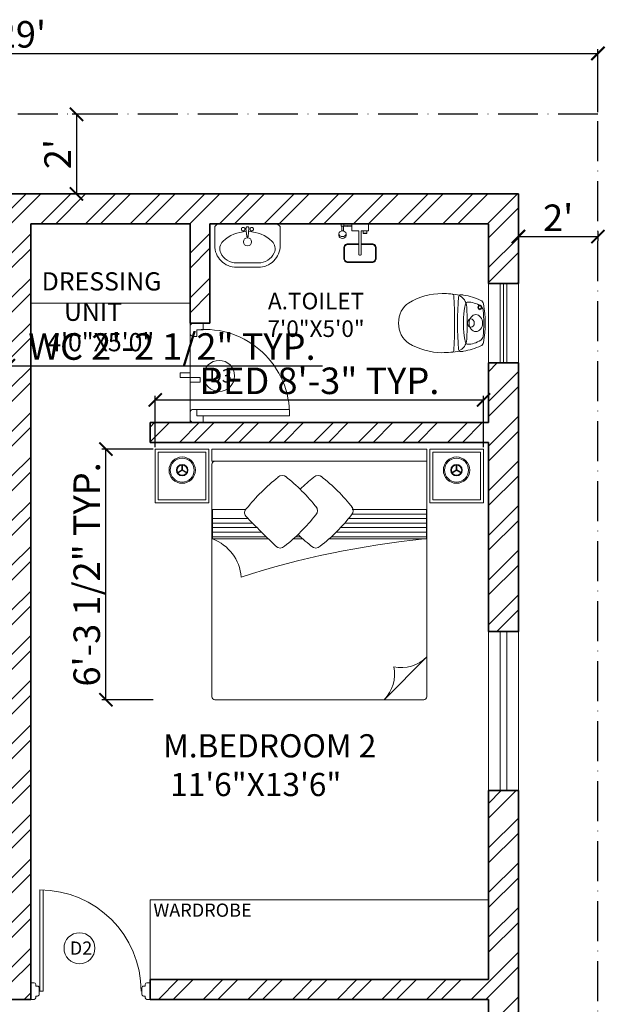
# Model space of a CAD drawing. Units: inches. Extents: x -15 to 1053, y -1 to 793.
# Tile 8 of 8: x 793 to 969, y 496 to 793. Entities that reach past the tile are written whole.
import ezdxf

# ---------------------------------------------------------------- set-up
doc = ezdxf.new("R2010")
doc.units = ezdxf.units.IN
doc.linetypes.add('ACAD_ISO10W100', pattern=[18, 12, -3, 0, -3])
for name, color, linetype, lineweight in [('00 FURNITURE', 15, 'Continuous', 15), ('A-ANNO-DIMS', 2, 'Continuous', 18), ('A-ANNO-TEXT', 7, 'Continuous', 18), ('A-AREA-IDEN', 7, 'Continuous', 18), ('A-DOOR', 4, 'Continuous', 18), ('A-FLOR-CASE', 5, 'Continuous', 18), ('A-FLOR-FIXT', 8, 'Continuous', 13), ('A-FURN', 8, 'Continuous', 13), ('A-GLAZ', 4, 'Continuous', 18), ('A-WALL', 7, 'Continuous', 35), ('A-WALL-PATT', 8, 'Continuous', 13), ('A_FUR 1', 5, 'Continuous', 5), ('C-PROP', 1, 'ACAD_ISO10W100', 25)]:
    doc.layers.add(name, color=color, linetype=linetype, lineweight=lineweight)
doc.styles.add('1-100DIM', font='txt', dxfattribs={"height": 0.3})
doc.styles.get("Standard").update_dxf_attribs({"font": 'arial.ttf'})
doc.dimstyles.new('ISO-25', dxfattribs={"dimtxt": 8, "dimasz": 4, "dimexe": 1.25, "dimexo": 0.625, "dimtad": 1, "dimdec": 0, "dimlunit": 4, "dimtxsty": 'Standard', "dimblk": 'ARCHTICK', "dimcen": 3, "dimadec": 0, "dimazin": 0, "dimtfac": 1, "dimtdec": 0, "dimtmove": 0, "dimatfit": 3, "dimldrblk": 'ARCHTICK', "dimfxl": 1, "dimarcsym": 0})

# ---------------------------------------------------------------- blocks, each defined once
blk = doc.blocks.new('_ArchTick')
at = {"color": 0, "linetype": 'ByBlock', "const_width": 0.15}
blk.add_lwpolyline([(-0.5, -0.5), (0.5, 0.5)], dxfattribs=at)
blk = doc.blocks.new('*D18')
at = {"layer": 'A-ANNO-DIMS', "color": 0, "lineweight": -2, "transparency": 16777216}
for p, q in [((619.07, 765.39), (619.07, 784.39)), ((967.07, 765.39), (967.07, 784.39)), ((619.07, 783.14), (967.07, 783.14))]:
    blk.add_line(p, q, dxfattribs=at)
at = {"layer": 'Defpoints', "color": 0, "transparency": 16777216}
for p in [(967.07, 783.14), (619.07, 764.76), (967.07, 764.76)]:
    blk.add_point(p, dxfattribs=at)
at = {"layer": 'A-ANNO-DIMS', "color": 0, "lineweight": -2, "transparency": 16777216, "xscale": 4, "yscale": 4, "zscale": 4, "rotation": 180}
blk.add_blockref('_ArchTick', (619.07, 783.14), dxfattribs=at)
at = {"layer": 'A-ANNO-DIMS', "color": 0, "lineweight": -2, "transparency": 16777216, "xscale": 4, "yscale": 4, "zscale": 4}
blk.add_blockref('_ArchTick', (967.07, 783.14), dxfattribs=at)
at = {"layer": 'A-ANNO-DIMS', "color": 0, "transparency": 16777216, "insert": (793.07, 787.85), "char_height": 8, "attachment_point": 5}
blk.add_mtext("29'", dxfattribs=at)
blk = doc.blocks.new('ESTSET')
at = {"layer": 'A_FUR 1'}
for p, q in [((-10.44, 4.1), (-10.44, 32.1)), ((-8.44, 4.1), (-8.44, 32.1)), ((-36.44, 6.1), (-36.44, 3.1)), ((-34.44, 6.1), (-36.44, 6.1)), ((-34.44, 4.1), (-34.44, 6.1)), ((-34.44, 4.1), (-34.44, 6.1)), ((-8.44, 4.1), (-8.44, 6.1)), ((-8.44, 6.1), (-6.44, 6.1)), ((-8.44, 4.1), (-8.44, 6.1)), ((-6.44, 6.1), (-6.44, 3.1)), ((-32.44, 4.1), (-34.44, 4.1)), ((-32.44, 4.1), (-34.44, 4.1)), ((-32.44, 3.1), (-32.44, 4.1)), ((-10.44, 3.1), (-10.44, 4.1)), ((-10.44, 4.1), (-8.44, 4.1)), ((-10.44, 4.1), (-8.44, 4.1)), ((-6.44, 2.1), (-36.44, 2.1)), ((-35.44, 2.1), (-33.44, 2.1)), ((-7.44, 2.1), (-9.44, 2.1))]:
    blk.add_line(p, q, dxfattribs=at)
for points in [[(-21.44, 2.1), (-18.67, 2.1), (-18.67, 5.1), (-20.06, 5.1)], [(-20.06, 5.1), (-20.06, -0.91)], [(-21.44, 2.1), (-21.44, -0.91), (-20.06, -0.91)]]:
    blk.add_lwpolyline(points, dxfattribs=at)
for centre, radius, start, end in [((-8.91, 6.46), 25.64, 88.9606, 185.2816), ((-35.44, 3.1), 1, 180, 270), ((-33.44, 3.1), 1, 270, 0), ((-9.44, 3.1), 1, 180, 270), ((-7.44, 3.1), 1, 270, 0)]:
    blk.add_arc(centre, radius, start, end, dxfattribs=at)
blk = doc.blocks.new('DDD')
at = {"layer": '00 FURNITURE'}
for p, q in [((-12579.77, -15859.53), (-12579.77, -15829.05)), ((-12578.77, -15859.53), (-12578.77, -15829.03)), ((-12612.02, -15857.03), (-12612.02, -15862.03)), ((-12611.02, -15857.03), (-12612.02, -15857.03)), ((-12610.52, -15858.03), (-12610.52, -15857.53)), ((-12577.52, -15858.03), (-12577.52, -15857.53)), ((-12577.02, -15857.03), (-12576.02, -15857.03)), ((-12576.02, -15857.03), (-12576.02, -15862.03)), ((-12610.52, -15861.53), (-12610.52, -15861.03)), ((-12578.77, -15859.53), (-12579.77, -15859.53)), ((-12577.52, -15861.53), (-12577.52, -15861.03)), ((-12612.02, -15862.03), (-12611.02, -15862.03)), ((-12576.02, -15862.03), (-12577.02, -15862.03))]:
    blk.add_line(p, q, dxfattribs=at)
for points in [[(-12610.52, -15861.03), (-12610.02, -15861.03, 0.414214), (-12609.52, -15860.53), (-12609.52, -15858.53, 0.414214), (-12610.02, -15858.03), (-12610.52, -15858.03)], [(-12577.52, -15861.03), (-12578.02, -15861.03, -0.414214), (-12578.52, -15860.53), (-12578.52, -15858.53, -0.414214), (-12578.02, -15858.03), (-12577.52, -15858.03)]]:
    blk.add_lwpolyline(points, format="xyb", dxfattribs=at)
for centre, radius, start, end in [((-12578.77, -15859.53), 30.5, 90, 180), ((-12611.02, -15857.53), 0.5, 0, 90), ((-12577.02, -15857.53), 0.5, 90, 180), ((-12611.02, -15861.53), 0.5, 270, 0), ((-12577.02, -15861.53), 0.5, 180, 270)]:
    blk.add_arc(centre, radius, start, end, dxfattribs=at)
blk = doc.blocks.new('RGWTG')
at = {"layer": '00 FURNITURE'}
for p, q in [((578.23, 3473.51), (577.36, 3475.01)), ((578.23, 3473.58), (577.36, 3472.08)), ((578.36, 3473.58), (577.49, 3475.09)), ((578.36, 3473.51), (577.49, 3472)), ((578.29, 3473.62), (580.03, 3473.62)), ((578.29, 3473.47), (580.03, 3473.47)), ((521.93, 3464.58), (509.03, 3451.68)), ((509.03, 3422.63), (509.03, 3463.68)), ((509.93, 3464.58), (566.4, 3464.58)), ((557.53, 3463.84), (557.53, 3464.49)), ((557.53, 3464.49), (566.4, 3464.49)), ((558.2, 3464.49), (558.2, 3435.82)), ((559.57, 3464.49), (559.57, 3437.25)), ((560.94, 3464.49), (560.94, 3438.58)), ((562.3, 3464.49), (562.3, 3439.83)), ((563.67, 3464.49), (563.67, 3440.99)), ((565.04, 3464.49), (565.04, 3442.08)), ((566.4, 3464.58), (580.98, 3464.58)), ((566.4, 3464.49), (566.4, 3442.08)), ((566.4, 3464.49), (566.4, 3463.84)), ((580.98, 3464.58), (580.98, 3416.72)), ((558.2, 3426.48), (558.2, 3425.04)), ((509.03, 3400.68), (509.03, 3422.63)), ((558.2, 3416.13), (558.2, 3399.95)), ((580.98, 3416.72), (580.98, 3400.68)), ((559.57, 3414.75), (559.57, 3399.95)), ((560.94, 3413.39), (560.94, 3399.95)), ((562.3, 3412.04), (562.3, 3399.95)), ((563.67, 3410.72), (563.67, 3399.95)), ((580.08, 3399.78), (509.93, 3399.78)), ((557.53, 3399.95), (557.53, 3400.6)), ((566.4, 3399.95), (557.53, 3399.95)), ((566.4, 3400.6), (566.4, 3399.95)), ((578.23, 3390.78), (577.36, 3392.29)), ((578.36, 3390.86), (577.49, 3392.36)), ((578.23, 3390.86), (577.36, 3389.36)), ((578.36, 3390.78), (577.49, 3389.28)), ((578.29, 3390.9), (580.03, 3390.9)), ((578.29, 3390.74), (580.03, 3390.74))]:
    blk.add_line(p, q, dxfattribs=at)
for points in [[(568.43, 3465.48), (584.63, 3465.48), (584.63, 3481.68), (568.43, 3481.68)], [(569.33, 3466.38), (583.73, 3466.38), (583.73, 3480.78), (569.33, 3480.78)], [(580.98, 3399.78), (584.63, 3399.78), (584.63, 3464.58), (580.98, 3464.58)], [(568.43, 3398.88), (584.63, 3398.88), (584.63, 3382.68), (568.43, 3382.68)], [(569.33, 3397.98), (583.73, 3397.98), (583.73, 3383.58), (569.33, 3383.58)]]:
    blk.add_lwpolyline(points, close=True, dxfattribs=at)
for points in [[(566.52, 3464.49), (557.53, 3464.49), (557.53, 3435.08)], [(557.53, 3427.21), (557.53, 3424.3)], [(557.53, 3416.82), (557.53, 3399.95), (566.4, 3399.95), (566.4, 3409.94)]]:
    blk.add_lwpolyline(points, dxfattribs=at)
for centre, radius in [((578.29, 3473.54), 3.97), ((578.29, 3473.54), 3.63), ((578.29, 3473.54), 1.74), ((578.29, 3473.54), 1.56), ((578.29, 3390.82), 3.97), ((578.29, 3390.82), 3.63), ((578.29, 3390.82), 1.74), ((578.29, 3390.82), 1.56)]:
    blk.add_circle(centre, radius, dxfattribs=at)
for centre, radius, start, end in [((509.93, 3463.68), 0.9, 90, 180), ((529.65, 3456.88), 10.9, 135.0361, 191.9278), ((290.56, 3490.52), 268.3, 342.2214, 354.2925), ((516.73, 3443.97), 10.9, 78.0722, 134.9639), ((598.15, 3399.01), 54.32, 127.931, 142.069), ((566.05, 3440.57), 1.82, 45, 135), ((533.58, 3399.31), 54.32, 37.931, 52.069), ((556.59, 3431.11), 1.82, 135, 225), ((598.15, 3388.23), 54.32, 127.931, 142.069), ((566.05, 3429.78), 1.82, 45, 135), ((533.58, 3388.53), 54.32, 37.931, 52.069), ((574.84, 3431.77), 1.82, 315, 45), ((597.87, 3463.6), 54.32, 217.931, 224.141), ((533.28, 3463.88), 54.32, 316.32, 322.069), ((574.84, 3420.99), 1.82, 315, 45), ((556.59, 3420.33), 1.82, 135, 225), ((765.33, 3619.75), 290.45, 223.6069, 226.2326), ((533.28, 3453.1), 54.32, 307.931, 322.069), ((565.44, 3411.05), 1.47, 225.9674, 326.8337), ((545.02, 3395.29), 13.35, 20.4224, 85.5825), ((509.93, 3400.68), 0.9, 180, 270), ((580.08, 3400.68), 0.9, 270, 0)]:
    blk.add_arc(centre, radius, start, end, dxfattribs=at)
blk = doc.blocks.new('s_14')
at = {"extrusion": (0, 0, -1)}
for centre, major_axis, start_param, end_param in [((-0.2, -522.3), (652.4, -0.3), 4.476887, 4.947891), ((-0.2, -522.3), (652.4, -0.3), 4.476887, 4.947891), ((681.3, -278.7), (913.7, -0.4), 3.289642, 3.481728), ((681.3, -278.7), (913.7, -0.4), 3.289642, 3.481728), ((-143.1, -44.8), (39.1, 0), 3.481728, 4.476887), ((-143.1, -44.8), (39.1, 0), 3.481728, 4.476887), ((118.1, -139.4), (284.9, -0.1), 3.130806, 3.616946), ((-125.1, -42.1), (19.2, 0), 3.141593, 9.424778), ((-125.1, -42.1), (12.2, 0), 3.141593, 9.424778), ((-97.4, -50.5), (42.5, 0), 3.616946, 4.577347), ((-0.3, -624.1), (765.5, -0.4), 4.577347, 4.847431), ((0, -73.8), (67.1, 0), 3.141593, 9.424778), ((97.3, -50.6), (42.5, 0), -1.435755, -0.475353), ((-118.3, -139.3), (284.9, -0.1), -0.475353, 0.010787), ((143.1, -44.9), (39.1, 0), -1.335294, -0.340135), ((143.1, -44.9), (39.1, 0), -1.335294, -0.340135), ((-681.5, -278.1), (913.7, -0.4), -0.340135, -0.148049), ((-681.5, -278.1), (913.7, -0.4), -0.340135, -0.148049), ((-120.9, -224.6), (98.7, 0), 3.365215, 4.657014), ((-148.9, -141.6), (17.9, 0), 1.839297, 3.130806), ((0.1, 291.4), (579, -0.3), 1.302296, 1.839297), ((-0.9, -1969.6), (2281.8, -1.1), 4.657014, 4.767764), ((-0.1, -112.6), (32.9, 0), 3.141593, 9.424778), ((120.7, -224.8), (98.7, 0), -1.515421, -0.223622), ((148.8, -141.7), (17.9, 0), 0.010787, 1.302296), ((999.2, -341.8), (1233.1, -0.6), 3.141593, 3.282422), ((999.2, -341.8), (1233.1, -0.6), 3.141593, 3.282422), ((-87.1, -186.6), (136.8, -0.1), 3.032389, 3.289642), ((-87.1, -186.6), (136.8, -0.1), 3.032389, 3.289642), ((-207.2, -197.1), (16, 0), 1.680926, 3.032389), ((-207.2, -197.1), (16, 0), 1.680926, 3.032389), ((0.6, 1302.1), (1900.3, -0.9), 1.460666, 1.680926), ((0.6, 1302.1), (1900.3, -0.9), 1.460666, 1.680926), ((207, -197.3), (16, 0), 0.109204, 1.460666), ((207, -197.3), (16, 0), 0.109204, 1.460666), ((-999.6, -340.9), (1233.1, -0.6), -0.140829, 0), ((-999.6, -340.9), (1233.1, -0.6), -0.140829, 0), ((86.9, -186.7), (136.8, -0.1), -0.148049, 0.109204), ((86.9, -186.7), (136.8, -0.1), -0.148049, 0.109204), ((-210, -262.6), (19.7, 0), 3.222651, 4.658459), ((-1.6, -3375.8), (3914.3, -1.8), 4.658459, 4.766319), ((209.8, -262.8), (19.7, 0), -1.516867, -0.081058), ((526.7, -341.6), (760.5, -0.4), 2.693443, 3.141593), ((526.7, -341.6), (760.5, -0.4), 2.693443, 3.141593), ((-527, -341.1), (760.5, -0.4), 0, 0.44815), ((-527, -341.1), (760.5, -0.4), 0, 0.44815), ((-0.3, -544.1), (175.9, -0.1), 0.44815, 2.693443), ((-0.3, -544.1), (175.9, -0.1), 0.44815, 2.693443)]:
    blk.add_ellipse(centre, major_axis=major_axis, ratio=0.800511, start_param=start_param, end_param=end_param, dxfattribs=at)
blk = doc.blocks.new('s_46')
at = {"ltscale": 600}
h = blk.add_hatch(color=256, dxfattribs=at)
edge = h.paths.add_edge_path()
edge.add_line((13.5, 62), (14.2, 54.1))
edge.add_ellipse((4.2, 52.3), major_axis=(-10.1, 0), ratio=1, start_angle=540, end_angle=550.17546, ccw=False)
edge.add_arc((4.2, 52.3), 10.1, 270, 360, ccw=False)
edge.add_line((4.2, 42.2), (4.2, 41.3))
edge.add_line((4.2, 41.3), (11.9, 41.3))
edge.add_arc((4.2, 52.3), 13.4, 664.69813, 766.48477)
h.paths.add_polyline_path([(4.2, 41.3), (-3.4, 41.3, 0.152567), (4.2, 38.9)])
h.paths.add_polyline_path([(11.9, 41.3), (4.2, 41.3), (4.2, 38.9, 0.152567)])
h.paths.add_polyline_path([(-5.7, 54.1), (-5, 62, 0.475833), (-3.4, 41.3), (4.2, 41.3), (4.2, 42.2, -0.46724)])
for p, q in [((-5.9, 52.3), (-0.7, 110.5)), ((-5.9, 52.3), (-0.7, 110.5)), ((9.1, 110.5), (14.2, 54.1)), ((14.3, 52.3), (9.1, 110.5)), ((14.2, 54.1), (14.3, 52.3))]:
    blk.add_line(p, q, dxfattribs=at)
blk.add_lwpolyline([(-220.8, 171.3, -0.414214), (-70.8, 321.3), (79.2, 321.3, -0.414214), (229.2, 171.3), (229.2, 41.3), (209.2, 21.3), (-200.8, 21.3), (-220.8, 41.3)], format="xyb", close=True, dxfattribs=at)
blk.add_lwpolyline([(12.3, 75.4, 0.181638), (172.2, 141.5, 0.326351), (187.7, 222.7, 0.289814), (79.2, 291.3), (-70.8, 291.3, 0.289814), (-179.2, 222.7, 0.326351), (-163.8, 141.5, 0.181638), (-3.8, 75.4)], format="xyb", dxfattribs=at)
for points in [[(-16.8, 67.4), (-17, 67.5), (-17.2, 67.6), (-17.4, 67.6), (-17.6, 67.7), (-17.8, 67.8), (-18, 67.9), (-18.1, 68.1), (-18.2, 68.2), (-18.3, 68.4), (-18.4, 68.6), (-18.5, 68.8), (-18.7, 68.9), (-18.8, 69.1), (-18.9, 69.2), (-19.1, 69.3), (-19.3, 69.3), (-19.5, 69.3), (-19.7, 69.4), (-19.9, 69.4), (-20.1, 69.4), (-20.3, 69.4), (-20.5, 69.5), (-20.7, 69.6), (-20.8, 69.7), (-21, 69.9), (-21.1, 70), (-21.3, 70.2), (-21.4, 70.3), (-21.5, 70.4), (-21.7, 70.5), (-21.9, 70.5), (-22.1, 70.5), (-22.3, 70.5), (-22.5, 70.5), (-22.7, 70.4), (-22.9, 70.4), (-23.1, 70.4), (-23.3, 70.4), (-23.5, 70.5), (-23.7, 70.6), (-23.9, 70.7), (-24, 70.8), (-24.2, 70.9), (-24.4, 71), (-24.6, 71.1), (-24.7, 71.1), (-24.9, 71.1), (-25.1, 71), (-25.3, 71), (-25.5, 70.9), (-25.7, 70.8), (-25.9, 70.7), (-26.1, 70.6), (-26.3, 70.6), (-26.5, 70.6), (-26.7, 70.6), (-26.9, 70.7), (-27.1, 70.8), (-27.3, 70.8), (-27.5, 70.9), (-27.7, 70.9), (-27.8, 70.9), (-28, 70.8), (-28.2, 70.8), (-28.3, 70.6), (-28.5, 70.5), (-28.7, 70.4), (-28.9, 70.3), (-29.1, 70.2), (-29.3, 70.1), (-29.6, 70.1), (-29.9, 70.1), (-30.2, 70.1), (-30.5, 70), (-30.8, 69.8), (-31.1, 69.5), (-31.4, 69), (-31.6, 68.4), (-32.3, 68.5), (-32.8, 68.4), (-33.2, 68.3), (-33.5, 68.1), (-33.7, 67.8), (-33.9, 67.6), (-34, 67.3), (-34.1, 67.1), (-34.3, 66.9), (-34.5, 66.7), (-34.7, 66.6), (-34.9, 66.5), (-35.1, 66.4), (-35.2, 66.3), (-35.4, 66.2), (-35.5, 66), (-35.6, 65.9), (-35.6, 65.7), (-35.7, 65.5), (-35.7, 65.3), (-35.7, 65.1), (-35.8, 64.9), (-35.8, 64.7), (-35.9, 64.5), (-36, 64.3), (-36.2, 64.2), (-36.3, 64), (-36.5, 63.9), (-36.6, 63.8), (-36.8, 63.6), (-36.9, 63.5), (-37, 63.3), (-37, 63.1), (-37, 63), (-37, 62.8), (-37, 62.6), (-37, 62.3), (-37, 62.1), (-37, 61.9), (-37, 61.7), (-37.1, 61.5), (-37.2, 61.4), (-37.3, 61.2), (-37.4, 61), (-37.5, 60.8), (-37.6, 60.7), (-37.7, 60.5), (-37.8, 60.3), (-37.8, 60.1), (-37.7, 60), (-37.7, 59.8), (-37.6, 59.6), (-37.5, 59.4), (-37.4, 59.2), (-37.4, 59), (-37.4, 58.8), (-37.4, 58.6), (-37.4, 58.4), (-37.5, 58.2), (-37.6, 58), (-37.7, 57.8), (-37.7, 57.6), (-37.8, 57.4), (-37.8, 57.2), (-37.7, 57.1), (-37.6, 56.9), (-37.5, 56.7), (-37.4, 56.6), (-37.3, 56.4), (-37.2, 56.2), (-37.1, 56), (-37, 55.8), (-37, 55.6), (-37, 55.4), (-37, 55.2), (-37, 55), (-37, 54.8), (-37, 54.6), (-37, 54.4), (-37, 54.2), (-36.9, 54.1), (-36.8, 53.9), (-36.6, 53.8), (-36.5, 53.7), (-36.3, 53.5), (-36.2, 53.4), (-36, 53.2), (-35.9, 53.1), (-35.8, 52.9), (-35.8, 52.7), (-35.7, 52.5), (-35.7, 52.3), (-35.7, 52.1), (-35.6, 51.9), (-35.6, 51.7), (-35.5, 51.5), (-35.4, 51.4), (-35.2, 51.3), (-35.1, 51.2), (-34.9, 51.1), (-34.7, 51), (-34.5, 50.9), (-34.3, 50.8), (-34.2, 50.7), (-34, 50.5), (-33.9, 50.3), (-33.8, 50.1), (-33.8, 49.9), (-33.7, 49.8), (-33.6, 49.6), (-33.5, 49.4), (-33.4, 49.3), (-33.2, 49.2), (-33.1, 49.1), (-32.9, 49.1), (-32.7, 49), (-32.5, 49), (-32.2, 48.9), (-32.1, 48.9), (-31.9, 48.8), (-31.7, 48.7), (-31.6, 48.5), (-31.4, 48.3), (-31.3, 48.2), (-31.2, 48), (-31.1, 47.9), (-30.9, 47.7), (-30.8, 47.6), (-30.6, 47.6), (-30.4, 47.5), (-30.2, 47.5), (-30, 47.6), (-29.8, 47.6), (-29.6, 47.6), (-29.4, 47.6), (-29.2, 47.5), (-29, 47.4), (-28.8, 47.3), (-28.7, 47.2), (-28.5, 47.1), (-28.3, 46.9), (-28.2, 46.8), (-28, 46.7), (-27.8, 46.7), (-27.7, 46.7), (-27.5, 46.7), (-27.3, 46.7), (-27.1, 46.8), (-26.9, 46.9), (-26.7, 46.9), (-26.5, 47), (-26.3, 47), (-26.1, 46.9), (-25.9, 46.9), (-25.7, 46.8), (-25.5, 46.7), (-25.3, 46.6), (-25.1, 46.5), (-24.9, 46.5), (-24.7, 46.5), (-24.6, 46.5), (-24.4, 46.6), (-24.2, 46.7), (-24, 46.8), (-23.9, 46.9), (-23.7, 47), (-23.5, 47.1), (-23.3, 47.1), (-23.1, 47.2), (-22.9, 47.2), (-22.7, 47.1), (-22.5, 47.1), (-22.3, 47), (-22.1, 47), (-21.9, 47), (-21.7, 47.1), (-21.5, 47.1), (-21.4, 47.2), (-21.3, 47.4), (-21.1, 47.5), (-21, 47.7), (-20.8, 47.8), (-20.7, 48), (-20.5, 48.1), (-20.3, 48.1), (-20.1, 48.2), (-19.9, 48.2), (-19.7, 48.2), (-19.5, 48.2), (-19.3, 48.2), (-19.1, 48.3), (-18.9, 48.4), (-18.8, 48.5), (-18.7, 48.6), (-18.5, 48.8), (-18.4, 49), (-18.3, 49.2), (-18.2, 49.3), (-18.1, 49.5), (-18, 49.7), (-17.8, 49.8), (-17.6, 49.9), (-17.4, 49.9), (-17.2, 50), (-17, 50.1), (-16.8, 50.1), (-16.7, 50.2), (-16.5, 50.3), (-16.4, 50.5), (-16.3, 50.7), (-16.3, 50.8), (-16.2, 51), (-16.2, 51.3), (-16.1, 51.5), (-16, 51.6), (-15.9, 51.8), (-15.8, 52), (-15.6, 52.1), (-15.5, 52.2), (-15.3, 52.3), (-15.1, 52.4), (-15, 52.6), (-14.8, 52.7), (-14.7, 52.8), (-14.7, 53), (-14.6, 53.2), (-14.6, 53.4), (-14.6, 53.6), (-14.6, 53.8), (-14.6, 54), (-14.6, 54.2), (-14.5, 54.4), (-14.4, 54.6), (-14.3, 54.8), (-14.2, 54.9), (-14, 55.1), (-13.9, 55.2), (-13.7, 55.4), (-13.6, 55.5), (-13.6, 55.7), (-13.6, 55.9), (-13.6, 56.1), (-13.6, 56.3), (-13.7, 56.5), (-13.7, 56.7), (-13.8, 56.9), (-13.8, 57.1), (-13.8, 57.3), (-13.7, 57.5), (-13.7, 57.7), (-13.6, 57.9), (-13.5, 58.1), (-13.4, 58.2), (-13.3, 58.4), (-13.2, 58.6), (-13.2, 58.8), (-13.2, 59), (-13.3, 59.1), (-13.4, 59.3), (-13.5, 59.5), (-13.6, 59.7), (-13.7, 59.9), (-13.7, 60.1), (-13.8, 60.3), (-13.8, 60.5), (-13.8, 60.7), (-13.7, 60.9), (-13.7, 61.1), (-13.6, 61.3), (-13.6, 61.5), (-13.6, 61.7), (-13.6, 61.9), (-13.6, 62), (-13.7, 62.2), (-13.9, 62.3), (-14, 62.5), (-14.2, 62.6), (-14.3, 62.8), (-14.4, 63), (-14.5, 63.1), (-14.6, 63.3), (-14.6, 63.5), (-14.6, 63.8), (-14.6, 64), (-14.6, 64.2), (-14.6, 64.4), (-14.7, 64.6), (-14.7, 64.7), (-14.8, 64.9), (-15, 65), (-15.1, 65.1), (-15.3, 65.2), (-15.5, 65.3), (-15.6, 65.5), (-15.8, 65.6), (-15.9, 65.7), (-16, 65.9), (-16.1, 66.1), (-16.2, 66.3), (-16.2, 66.5), (-16.3, 66.7), (-16.3, 66.9), (-16.4, 67.1), (-16.5, 67.2), (-16.7, 67.3)], [(22.1, 61.1), (22, 61.3), (22, 61.5), (22, 61.7), (22, 61.9), (22.1, 62), (22.2, 62.2), (22.3, 62.3), (22.4, 62.5), (22.6, 62.6), (22.7, 62.8), (22.8, 63), (22.9, 63.1), (23, 63.3), (23, 63.5), (23, 63.8), (23, 64), (23, 64.2), (23, 64.4), (23.1, 64.6), (23.1, 64.7), (23.2, 64.9), (23.4, 65), (23.5, 65.1), (23.7, 65.2), (23.9, 65.3), (24.1, 65.5), (24.2, 65.6), (24.4, 65.7), (24.5, 65.9), (24.5, 66.1), (24.6, 66.3), (24.7, 66.5), (24.7, 66.7), (24.8, 66.9), (24.9, 67.1), (25, 67.2), (25.1, 67.3), (25.3, 67.4), (25.4, 67.5), (25.6, 67.6), (25.8, 67.6), (26, 67.7), (26.2, 67.8), (26.4, 67.9), (26.5, 68.1), (26.7, 68.2), (26.8, 68.4), (26.9, 68.6), (27, 68.8), (27.1, 68.9), (27.2, 69.1), (27.3, 69.2), (27.5, 69.3), (27.7, 69.3), (27.9, 69.3), (28.1, 69.4), (28.3, 69.4), (28.5, 69.4), (28.7, 69.4), (28.9, 69.5), (29.1, 69.6), (29.2, 69.7), (29.4, 69.9), (29.5, 70), (29.7, 70.2), (29.8, 70.3), (30, 70.4), (30.1, 70.5), (30.3, 70.5), (30.5, 70.5), (30.7, 70.5), (30.9, 70.5), (31.1, 70.4), (31.3, 70.4), (31.5, 70.4), (31.7, 70.4), (31.9, 70.5), (32.1, 70.6), (32.3, 70.7), (32.5, 70.8), (32.6, 70.9), (32.8, 71), (33, 71.1), (33.2, 71.1), (33.4, 71.1), (33.5, 71), (33.7, 71), (33.9, 70.9), (34.1, 70.8), (34.3, 70.7), (34.5, 70.6), (34.7, 70.6), (34.9, 70.6), (35.1, 70.6), (35.3, 70.7), (35.5, 70.8), (35.7, 70.8), (35.9, 70.9), (36.1, 70.9), (36.3, 70.9), (36.4, 70.8), (36.6, 70.8), (36.8, 70.6), (36.9, 70.5), (37.1, 70.4), (37.3, 70.3), (37.5, 70.2), (37.8, 70.1), (38, 70.1), (38.3, 70.1), (38.6, 70.1), (38.9, 70), (39.2, 69.8), (39.5, 69.5), (39.8, 69), (40.1, 68.4), (40.7, 68.5), (41.3, 68.4), (41.7, 68.3), (42, 68.1), (42.2, 67.8), (42.3, 67.6), (42.4, 67.3), (42.6, 67.1), (42.7, 66.9), (42.9, 66.7), (43.1, 66.6), (43.3, 66.5), (43.5, 66.4), (43.6, 66.3), (43.8, 66.2), (43.9, 66), (44, 65.9), (44.1, 65.7), (44.1, 65.5), (44.1, 65.3), (44.2, 65.1), (44.2, 64.9), (44.2, 64.7), (44.3, 64.5), (44.4, 64.3), (44.6, 64.2), (44.7, 64), (44.9, 63.9), (45.1, 63.8), (45.2, 63.6), (45.3, 63.5), (45.4, 63.3), (45.5, 63.1), (45.5, 63), (45.5, 62.8), (45.4, 62.6), (45.4, 62.3), (45.4, 62.1), (45.4, 61.9), (45.4, 61.7), (45.5, 61.5), (45.6, 61.4), (45.7, 61.2), (45.8, 61), (46, 60.8), (46.1, 60.7), (46.1, 60.5), (46.2, 60.3), (46.2, 60.1), (46.1, 60), (46.1, 59.8), (46, 59.6), (45.9, 59.4), (45.9, 59.2), (45.8, 59), (45.8, 58.8), (45.8, 58.6), (45.9, 58.4), (45.9, 58.2), (46, 58), (46.1, 57.8), (46.1, 57.6), (46.2, 57.4), (46.2, 57.2), (46.1, 57.1), (46.1, 56.9), (46, 56.7), (45.8, 56.6), (45.7, 56.4), (45.6, 56.2), (45.5, 56), (45.4, 55.8), (45.4, 55.6), (45.4, 55.4), (45.4, 55.2), (45.4, 55), (45.5, 54.8), (45.5, 54.6), (45.5, 54.4), (45.4, 54.2), (45.3, 54.1), (45.2, 53.9), (45.1, 53.8), (44.9, 53.7), (44.7, 53.5), (44.6, 53.4), (44.4, 53.2), (44.3, 53.1), (44.2, 52.9), (44.2, 52.7), (44.2, 52.5), (44.1, 52.3), (44.1, 52.1), (44.1, 51.9), (44, 51.7), (43.9, 51.5), (43.8, 51.4), (43.6, 51.3), (43.5, 51.2), (43.3, 51.1), (43.1, 51), (42.9, 50.9), (42.7, 50.8), (42.6, 50.7), (42.5, 50.5), (42.4, 50.3), (42.3, 50.1), (42.2, 49.9), (42.1, 49.8), (42, 49.6), (41.9, 49.4), (41.8, 49.3), (41.7, 49.2), (41.5, 49.1), (41.3, 49.1), (41.1, 49), (40.9, 49), (40.7, 48.9), (40.5, 48.9), (40.3, 48.8), (40.1, 48.7), (40, 48.5), (39.9, 48.3), (39.7, 48.2), (39.6, 48), (39.5, 47.9), (39.4, 47.7), (39.2, 47.6), (39, 47.6), (38.8, 47.5), (38.6, 47.5), (38.4, 47.6), (38.2, 47.6), (38, 47.6), (37.8, 47.6), (37.6, 47.5), (37.4, 47.4), (37.2, 47.3), (37.1, 47.2), (36.9, 47.1), (36.8, 46.9), (36.6, 46.8), (36.4, 46.7), (36.3, 46.7), (36.1, 46.7), (35.9, 46.7), (35.7, 46.7), (35.5, 46.8), (35.3, 46.9), (35.1, 46.9), (34.9, 47), (34.7, 47), (34.5, 46.9), (34.3, 46.9), (34.1, 46.8), (33.9, 46.7), (33.7, 46.6), (33.5, 46.5), (33.4, 46.5), (33.2, 46.5), (33, 46.5), (32.8, 46.6), (32.6, 46.7), (32.5, 46.8), (32.3, 46.9), (32.1, 47), (31.9, 47.1), (31.7, 47.1), (31.5, 47.2), (31.3, 47.2), (31.1, 47.1), (30.9, 47.1), (30.7, 47), (30.5, 47), (30.3, 47), (30.1, 47.1), (30, 47.1), (29.8, 47.2), (29.7, 47.4), (29.5, 47.5), (29.4, 47.7), (29.2, 47.8), (29.1, 48), (28.9, 48.1), (28.7, 48.1), (28.5, 48.2), (28.3, 48.2), (28.1, 48.2), (27.9, 48.2), (27.7, 48.2), (27.5, 48.3), (27.3, 48.4), (27.2, 48.5), (27.1, 48.6), (27, 48.8), (26.9, 49), (26.8, 49.2), (26.7, 49.3), (26.5, 49.5), (26.4, 49.7), (26.2, 49.8), (26, 49.9), (25.8, 49.9), (25.6, 50), (25.4, 50.1), (25.3, 50.1), (25.1, 50.2), (25, 50.3), (24.9, 50.5), (24.8, 50.7), (24.7, 50.8), (24.7, 51), (24.6, 51.3), (24.5, 51.5), (24.5, 51.6), (24.4, 51.8), (24.2, 52), (24.1, 52.1), (23.9, 52.2), (23.7, 52.3), (23.5, 52.4), (23.4, 52.6), (23.2, 52.7), (23.1, 52.8), (23.1, 53), (23, 53.2), (23, 53.4), (23, 53.6), (23, 53.8), (23, 54), (23, 54.2), (22.9, 54.4), (22.8, 54.6), (22.7, 54.8), (22.6, 54.9), (22.4, 55.1), (22.3, 55.2), (22.2, 55.4), (22.1, 55.5), (22, 55.7), (22, 55.9), (22, 56.1), (22, 56.3), (22.1, 56.5), (22.1, 56.7), (22.2, 56.9), (22.2, 57.1), (22.2, 57.3), (22.2, 57.5), (22.1, 57.7), (22, 57.9), (21.9, 58.1), (21.8, 58.2), (21.7, 58.4), (21.6, 58.6), (21.6, 58.8), (21.6, 59), (21.7, 59.1), (21.8, 59.3), (21.9, 59.5), (22, 59.7), (22.1, 59.9), (22.2, 60.1), (22.2, 60.3), (22.2, 60.5), (22.2, 60.7), (22.1, 60.9)]]:
    blk.add_lwpolyline(points, close=True, dxfattribs=at)
blk.add_circle((4.2, 146.3), 28, dxfattribs=at)
for centre, radius, start, end in [((4.2, 108.2), 5.42, 24.6783, 155.3217), ((4.2, 52.3), 10.1, 169.82454, 0)]:
    blk.add_arc(centre, radius, start, end, dxfattribs=at)
for centre, major_axis, ratio, start_param, end_param in [((4.2, 110.5), (-4.93, 0), 0.641024, 3.141593, 6.283185), ((4.2, 52.3), (-10.1, 0), 1, 6.10559, 9.602373)]:
    blk.add_ellipse(centre, major_axis=major_axis, ratio=ratio, start_param=start_param, end_param=end_param, dxfattribs=at)
blk = doc.blocks.new('A$C7A0926BE')
for p, q in [((-6.55, 0), (-5.57, 0)), ((-6.55, -0.65), (-6.55, 0)), ((-5.57, 0), (-5.57, -0.65)), ((-2.89, 0), (-2.89, -2.29)), ((2.89, 0), (-2.89, 0)), ((2.89, -2.29), (2.89, 0)), ((-7.32, -3.29), (-7.32, -3.94)), ((-5.57, -0.65), (-6.55, -0.65)), ((-6.34, -0.65), (-5.74, -0.65)), ((-6.34, -2.33), (-6.34, -0.65)), ((-5.74, -2.33), (-6.34, -2.33)), ((-5.74, -0.65), (-5.74, -2.33)), ((-5.57, -0.28), (-2.89, -0.56)), ((-5.57, -0.65), (-2.89, -0.94)), ((-4.84, -3.94), (-4.85, -3.29)), ((-2.89, -2.29), (-0.45, -2.29)), ((0.39, -2.29), (2.89, -2.29)), ((1.04, -2.29), (1.04, -3.12)), ((2.37, -2.29), (1.04, -2.29)), ((1.04, -3.12), (2.37, -3.12)), ((1.13, -3.12), (1.13, -3.23)), ((2.3, -3.12), (1.13, -3.12)), ((1.13, -3.23), (2.3, -3.23)), ((2.3, -3.23), (2.3, -3.12)), ((2.37, -3.12), (2.37, -2.29))]:
    blk.add_line(p, q)
at = {"ltscale": 100}
for p, q in [((-0.45, -10.48), (-0.45, -2.29)), ((0.39, -10.48), (0.39, -2.29)), ((0.18, -10.69), (-0.24, -10.69))]:
    blk.add_line(p, q, dxfattribs=at)
for points in [[(-0.45, -6.79), (-4.23, -6.79, 0.414214), (-5.63, -8.19), (-5.63, -11.8, 0.414214), (-4.23, -13.2), (4.17, -13.2, 0.414214), (5.57, -11.8), (5.57, -8.19, 0.414214), (4.17, -6.79), (0.39, -6.79)], [(-0.45, -7), (-4.23, -7, 0.414214), (-5.42, -8.19), (-5.42, -11.8, 0.414214), (-4.23, -12.99), (4.17, -12.99, 0.414214), (5.36, -11.8), (5.36, -8.19, 0.414214), (4.17, -7), (0.39, -7)]]:
    blk.add_lwpolyline(points, format="xyb", dxfattribs=at)
for centre, start, end in [((-0.24, -10.48), 180, 270), ((0.18, -10.48), 270, 0)]:
    blk.add_arc(centre, 0.21, start, end, dxfattribs=at)
at = {"extrusion": (0, 0, -1)}
blk.add_ellipse((-6.08, -3.29), major_axis=(-1.24, 0), ratio=0.790849, dxfattribs=at)
blk.add_ellipse((-6.08, -3.94), major_axis=(-1.24, 0), ratio=0.790849, start_param=3.141593, end_param=6.283185, dxfattribs=at)
blk = doc.blocks.new('*D22')
at = {"layer": 'A-ANNO-DIMS', "color": 0, "lineweight": -2, "transparency": 16777216}
for p, q in [((810.21, 764.76), (808.57, 764.76)), ((809.82, 764.76), (809.82, 740.76)), ((810.21, 740.76), (808.57, 740.76))]:
    blk.add_line(p, q, dxfattribs=at)
at = {"layer": 'Defpoints', "color": 0, "transparency": 16777216}
for p in [(810.84, 764.76), (809.82, 740.76), (810.84, 740.76)]:
    blk.add_point(p, dxfattribs=at)
at = {"layer": 'A-ANNO-DIMS', "color": 0, "lineweight": -2, "transparency": 16777216, "xscale": 4, "yscale": 4, "zscale": 4}
for p, rotation in [((809.82, 764.76), 90), ((809.82, 740.76), 270)]:
    blk.add_blockref('_ArchTick', p, dxfattribs=dict(at, rotation=rotation))
at = {"layer": 'A-ANNO-DIMS', "color": 0, "transparency": 16777216, "insert": (805.18, 752.76), "char_height": 8, "attachment_point": 5, "rotation": 90}
blk.add_mtext("2'", dxfattribs=at)
blk = doc.blocks.new('*D23')
at = {"layer": 'A-ANNO-DIMS', "color": 0, "lineweight": -2, "transparency": 16777216}
for p, q in [((943.07, 729.37), (943.07, 726.62)), ((943.07, 727.87), (967.07, 727.87)), ((967.07, 729.37), (967.07, 726.62))]:
    blk.add_line(p, q, dxfattribs=at)
at = {"layer": 'Defpoints', "color": 0, "transparency": 16777216}
for p in [(943.07, 730), (967.07, 730), (967.07, 727.87)]:
    blk.add_point(p, dxfattribs=at)
at = {"layer": 'A-ANNO-DIMS', "color": 0, "lineweight": -2, "transparency": 16777216, "xscale": 4, "yscale": 4, "zscale": 4, "rotation": 180}
blk.add_blockref('_ArchTick', (943.07, 727.87), dxfattribs=at)
at = {"layer": 'A-ANNO-DIMS', "color": 0, "lineweight": -2, "transparency": 16777216, "xscale": 4, "yscale": 4, "zscale": 4}
blk.add_blockref('_ArchTick', (967.07, 727.87), dxfattribs=at)
at = {"layer": 'A-ANNO-DIMS', "color": 0, "transparency": 16777216, "insert": (955.07, 732.51), "char_height": 8, "attachment_point": 5}
blk.add_mtext("2'", dxfattribs=at)
blk = doc.blocks.new('*D38')
at = {"layer": 'A-ANNO-DIMS', "color": 0, "lineweight": -2, "transparency": 16777216}
for p, q in [((762.94, 692.23), (762.94, 687.66)), ((789.26, 692.23), (789.26, 687.66)), ((762.94, 688.91), (789.26, 688.91)), ((789.26, 688.91), (883.97, 688.91))]:
    blk.add_line(p, q, dxfattribs=at)
at = {"layer": 'Defpoints', "color": 0, "transparency": 16777216}
for p in [(762.94, 692.85), (789.26, 692.85), (789.26, 688.91)]:
    blk.add_point(p, dxfattribs=at)
at = {"layer": 'A-ANNO-DIMS', "color": 0, "lineweight": -2, "transparency": 16777216, "xscale": 4, "yscale": 4, "zscale": 4, "rotation": 180}
blk.add_blockref('_ArchTick', (762.94, 688.91), dxfattribs=at)
at = {"layer": 'A-ANNO-DIMS', "color": 0, "lineweight": -2, "transparency": 16777216, "xscale": 4, "yscale": 4, "zscale": 4}
blk.add_blockref('_ArchTick', (789.26, 688.91), dxfattribs=at)
at = {"layer": 'A-ANNO-DIMS', "color": 0, "transparency": 16777216, "insert": (838.61, 693.67), "char_height": 8, "attachment_point": 5}
blk.add_mtext('WC 2\'-2 1/2" TYP.', dxfattribs=at)
blk = doc.blocks.new('*D44')
at = {"layer": 'A-ANNO-DIMS', "color": 0, "lineweight": -2, "transparency": 16777216}
for p, q in [((833.57, 664.39), (833.57, 679.86)), ((833.57, 678.61), (932.57, 678.61)), ((932.57, 664.39), (932.57, 679.86))]:
    blk.add_line(p, q, dxfattribs=at)
at = {"layer": 'Defpoints', "color": 0, "transparency": 16777216}
for p in [(932.57, 678.61), (833.57, 663.76), (932.57, 663.76)]:
    blk.add_point(p, dxfattribs=at)
at = {"layer": 'A-ANNO-DIMS', "color": 0, "lineweight": -2, "transparency": 16777216, "xscale": 4, "yscale": 4, "zscale": 4, "rotation": 180}
blk.add_blockref('_ArchTick', (833.57, 678.61), dxfattribs=at)
at = {"layer": 'A-ANNO-DIMS', "color": 0, "lineweight": -2, "transparency": 16777216, "xscale": 4, "yscale": 4, "zscale": 4}
blk.add_blockref('_ArchTick', (932.57, 678.61), dxfattribs=at)
at = {"layer": 'A-ANNO-DIMS', "color": 0, "transparency": 16777216, "insert": (883.07, 683.33), "char_height": 8, "attachment_point": 5}
blk.add_mtext('BED 8\'-3" TYP.', dxfattribs=at)
blk = doc.blocks.new('*D45')
at = {"layer": 'A-ANNO-DIMS', "color": 0, "lineweight": -2, "transparency": 16777216}
for p, q in [((832.95, 663.76), (817.47, 663.76)), ((818.72, 588.16), (818.72, 663.76)), ((832.95, 588.16), (817.47, 588.16))]:
    blk.add_line(p, q, dxfattribs=at)
at = {"layer": 'Defpoints', "color": 0, "transparency": 16777216}
for p in [(818.72, 663.76), (833.57, 663.76), (833.57, 588.16)]:
    blk.add_point(p, dxfattribs=at)
at = {"layer": 'A-ANNO-DIMS', "color": 0, "lineweight": -2, "transparency": 16777216, "xscale": 4, "yscale": 4, "zscale": 4}
for p, rotation in [((818.72, 663.76), 90), ((818.72, 588.16), 270)]:
    blk.add_blockref('_ArchTick', p, dxfattribs=dict(at, rotation=rotation))
at = {"layer": 'A-ANNO-DIMS', "color": 0, "transparency": 16777216, "insert": (813.96, 625.96), "char_height": 8, "attachment_point": 5, "rotation": 90}
blk.add_mtext('6\'-3 1/2" TYP.', dxfattribs=at)

msp = doc.modelspace()

# ---------------------------------------------------------------- hatches: boundary and pattern name
at = {"layer": 'A-WALL-PATT'}
h = msp.add_hatch(dxfattribs=at)
h.set_pattern_fill('ANSI32', color=256)
h.paths.add_polyline_path([(754.07, 502.76), (754.07, 503.76), (652.07, 503.76), (652.07, 593.76), (643.07, 593.76), (643.07, 485.76), (652.07, 485.76), (652.07, 497.76), (754.07, 497.76)])
h.paths.add_polyline_path([(754.07, 449.76), (730.07, 449.76), (730.07, 467.76), (724.07, 467.76), (724.07, 449.76), (652.07, 449.76), (652.07, 461.76), (643.07, 461.76), (643.07, 374.76), (652.07, 374.76), (652.07, 443.76), (754.07, 443.76)])
h.paths.add_polyline_path([(757.07, 740.76), (643.07, 740.76), (643.07, 641.76), (652.07, 641.76), (652.07, 731.76), (700.07, 731.76), (700.07, 701.76), (706.07, 701.76), (706.07, 731.76), (757.07, 731.76)])
h.paths.add_polyline_path([(943.07, 740.76), (781.07, 740.76), (781.07, 731.76), (790.07, 731.76), (790.07, 671.76), (688.07, 671.76), (688.07, 665.76), (790.07, 665.76), (790.07, 497.76), (796.07, 497.76), (796.07, 502.76), (796.07, 731.76), (844.07, 731.76), (844.07, 701.76), (850.07, 701.76), (850.07, 731.76), (934.07, 731.76), (934.07, 713.76), (943.07, 713.76)])
h.paths.add_polyline_path([(943.07, 689.76), (934.07, 689.76), (934.07, 671.76), (832.07, 671.76), (832.07, 665.76), (934.07, 665.76), (934.07, 608.76), (943.07, 608.76)], flags=17)
h.paths.add_polyline_path([(943.07, 560.76), (934.07, 560.76), (934.07, 503.76), (832.07, 503.76), (832.07, 497.76), (934.07, 497.76), (934.07, 488.76), (943.07, 488.76)])
h.paths.add_polyline_path([(796.07, 449.76), (790.07, 449.76), (790.07, 444.76), (790.07, 326.76), (643.07, 326.76), (643.07, 320.76), (724.07, 320.76), (724.07, 266.76), (730.07, 266.76), (730.07, 320.76), (790.07, 320.76), (790.07, 272.76), (760.07, 272.76), (760.07, 266.76), (796.07, 266.76)])
h.paths.add_polyline_path([(652.07, 266.76), (688.07, 266.76), (688.07, 271.76), (688.07, 272.76), (643.07, 272.76), (643.07, 230.76), (652.07, 230.76)])
h.paths.add_polyline_path([(652.07, 182.76), (643.07, 182.76), (643.07, 146.76), (619.07, 146.76), (619.07, 44.76), (799.07, 44.76), (799.07, 53.76), (628.07, 53.76), (628.07, 137.76), (808.07, 137.76), (808.07, 146.76), (796.07, 146.76), (796.07, 218.76), (802.07, 218.76), (802.07, 224.76), (790.07, 224.76), (790.07, 146.76), (652.07, 146.76)])
h.paths.add_polyline_path([(886.07, 141.37), (886.07, 146.76), (850.07, 146.76), (850.07, 224.76), (838.07, 224.76), (838.07, 222.06), (838.07, 218.76), (844.07, 218.76), (844.07, 146.76), (832.07, 146.76), (832.07, 137.76), (886.07, 137.76)])
h.paths.add_polyline_path([(943.07, 176.76), (934.07, 176.76), (934.07, 137.76), (943.07, 137.76)])
h.paths.add_polyline_path([(943.07, 440.76), (934.07, 440.76), (934.07, 224.76), (943.07, 224.76)])

# ---------------------------------------------------------------- linework, layer by layer
at = {"layer": 'A-ANNO-TEXT'}
for centre in [(852.85, 685.85), (810.74, 513.2)]:
    msp.add_circle(centre, 4.67, dxfattribs=at)
at = {"layer": 'A-FLOR-CASE'}
for p, q in [((844.07, 707.76), (796.07, 707.76)), ((832.07, 503.76), (832.07, 527.76)), ((832.07, 527.76), (934.07, 527.76))]:
    msp.add_line(p, q, dxfattribs=at)
at = {"layer": 'A-GLAZ'}
for p, q in [((937.57, 689.76), (937.57, 713.76)), ((938.57, 689.76), (938.57, 713.76)), ((939.57, 689.76), (939.57, 713.76)), ((934.07, 608.76), (934.07, 560.76)), ((937.57, 608.76), (937.57, 560.76)), ((939.57, 608.76), (939.57, 560.76)), ((943.07, 608.76), (943.07, 560.76))]:
    msp.add_line(p, q, dxfattribs=at)
msp.add_lwpolyline([(943.07, 713.76), (934.07, 713.76), (934.07, 689.76), (943.07, 689.76)], close=True, dxfattribs=at)
at = {"layer": 'A-WALL'}
for p, q in [((943.07, 740.76), (781.07, 740.76)), ((943.07, 713.76), (943.07, 740.76)), ((796.07, 731.76), (796.07, 497.76)), ((844.07, 731.76), (796.07, 731.76)), ((844.07, 701.76), (844.07, 731.76)), ((934.07, 731.76), (850.07, 731.76)), ((850.07, 701.76), (850.07, 731.76)), ((934.07, 713.76), (934.07, 731.76)), ((934.07, 713.76), (943.07, 713.76)), ((850.07, 701.76), (844.07, 701.76)), ((934.07, 671.76), (934.07, 689.76)), ((934.07, 689.76), (943.07, 689.76)), ((943.07, 608.76), (943.07, 689.76)), ((934.07, 671.76), (832.07, 671.76)), ((832.07, 671.76), (832.07, 665.76)), ((934.07, 665.76), (832.07, 665.76)), ((934.07, 608.76), (934.07, 665.76)), ((934.07, 608.76), (943.07, 608.76)), ((934.07, 503.76), (934.07, 560.76)), ((934.07, 560.76), (943.07, 560.76)), ((943.07, 488.76), (943.07, 560.76)), ((934.07, 503.76), (832.07, 503.76)), ((832.07, 503.76), (832.07, 497.76)), ((790.07, 497.76), (796.07, 497.76)), ((934.07, 497.76), (832.07, 497.76)), ((934.07, 488.76), (934.07, 497.76))]:
    msp.add_line(p, q, dxfattribs=at)
at = {"layer": 'C-PROP'}
for p, q in [((967.07, 764.76), (619.07, 764.76)), ((967.07, 44.76), (967.07, 764.76))]:
    msp.add_line(p, q, dxfattribs=at)

# ---------------------------------------------------------------- block references
at = {"layer": 'A-DOOR', "rotation": 270}
msp.add_blockref('ESTSET', (841.98, 665.32), dxfattribs=at)
at = {"layer": 'A-DOOR', "xscale": -1}
msp.add_blockref('DDD', (-11779.95, 16359.79), dxfattribs=at)
at = {"layer": 'A-FLOR-FIXT'}
for name, p, xscale, yscale, zscale, rotation in [('s_46', (861.57, 732.7), 0.0438792252617072, 0.0438792252617072, 0.0438792252617072, 180), ('s_14', (933.07, 701.76), 0.0381558672165204, 0.0381558672165204, 0.0381558672165204, 270)]:
    msp.add_blockref(name, p, dxfattribs=dict(at, xscale=xscale, yscale=yscale, zscale=zscale, rotation=rotation))
at = {"layer": 'A-FLOR-FIXT', "extrusion": (0, 0, -1), "xscale": -0.8732967133751344, "yscale": 0.8732967133751344, "zscale": -0.8732967133751344}
msp.add_blockref('A$C7A0926BE', (-895.34, 731.61), dxfattribs=at)
at = {"layer": 'A-FURN', "xscale": -1, "rotation": 270}
msp.add_blockref('RGWTG', (-2549.11, 79.13), dxfattribs=at)

# ---------------------------------------------------------------- texts
at = {"layer": 'A-ANNO-TEXT', "char_height": 4, "attachment_point": 1}
for s, width, insert in [('D3', 8.4888, (849.9, 687.87)), ('WARDROBE', 23.2678, (833.02, 526.67)), ('D2', 8.4888, (807.8, 515.22))]:
    msp.add_mtext_dynamic_manual_height_columns(s, width=width, gutter_width=12.5, heights=[0], dxfattribs=dict(at, insert=insert))
at = {"layer": 'A-AREA-IDEN', "insert": (799.34, 717.11), "char_height": 8, "attachment_point": 1}
msp.add_mtext_dynamic_manual_height_columns('{\\H0.6875x;DRESSING\\P    UNIT\\P 4\'0"X5\'0" \\H1.18182x;    }  ', width=58.9878, gutter_width=0, heights=[37.04], dxfattribs=at)
at = {"layer": 'A-AREA-IDEN', "attachment_point": 1, "style": '1-100DIM'}
for s, width, insert, char_height in [('\\pxqc;{\\f@Malgun Gothic|b0|i0|c0|p34;A.TOILET\\P7\'0"X5\'0"}', 44.4016, (859.86, 710.93), 5), ('{\\f@Malgun Gothic|b0|i0|c0|p34;M.BEDROOM 2\\P 11\'6"X13\'6"}', 74.3652, (835.94, 577.75), 7)]:
    msp.add_mtext_dynamic_manual_height_columns(s, width=width, gutter_width=15.85, heights=[0], dxfattribs=dict(at, insert=insert, char_height=char_height))

# ---------------------------------------------------------------- dimensions: what is measured, and where the dimension line sits
at = {"layer": 'A-ANNO-DIMS'}
for base, p1, p2, picture, middle in [((967.07, 783.14), (619.07, 764.76), (967.07, 764.76), '*D18', (793.07, 787.85)), ((967.07, 727.87), (943.07, 730), (967.07, 730), '*D23', (955.07, 732.51))]:
    dim = msp.add_linear_dim(base=base, p1=p1, p2=p2, dimstyle='ISO-25', override={"dimclrd": 0, "dimclre": 0, "dimclrt": 0}, dxfattribs=at)
    dim.commit()
    dim.dimension.update_dxf_attribs({"geometry": picture, "text_midpoint": middle})
dim = msp.add_linear_dim(base=(809.82, 740.76), p1=(810.84, 764.76), p2=(810.84, 740.76), angle=90, dimstyle='ISO-25', override={"dimclrd": 0, "dimclre": 0, "dimclrt": 0}, dxfattribs=at)
dim.commit()
dim.dimension.update_dxf_attribs({"geometry": '*D22', "text_midpoint": (805.18, 752.76)})
for base, p1, p2, text, picture, middle in [((789.26, 688.91), (762.94, 692.85), (789.26, 692.85), 'WC <> TYP.', '*D38', (838.61, 693.67)), ((932.57, 678.61), (833.57, 663.76), (932.57, 663.76), 'BED <> TYP.', '*D44', (883.07, 683.33))]:
    dim = msp.add_linear_dim(base=base, p1=p1, p2=p2, text=text, dimstyle='ISO-25', override={"dimdec": 1, "dimrnd": 0, "dimzin": 1, "dimlunit": 4, "dimfrac": 2}, dxfattribs=at)
    dim.commit()
    dim.dimension.update_dxf_attribs({"geometry": picture, "text_midpoint": middle})
dim = msp.add_linear_dim(base=(818.72, 663.76), p1=(833.57, 588.16), p2=(833.57, 663.76), angle=90, text='<> TYP.', dimstyle='ISO-25', override={"dimdec": 1, "dimrnd": 0, "dimzin": 1, "dimlunit": 4, "dimfrac": 2}, dxfattribs=at)
dim.commit()
dim.dimension.update_dxf_attribs({"geometry": '*D45', "text_midpoint": (813.96, 625.96)})

doc.saveas('drawing.dxf')
